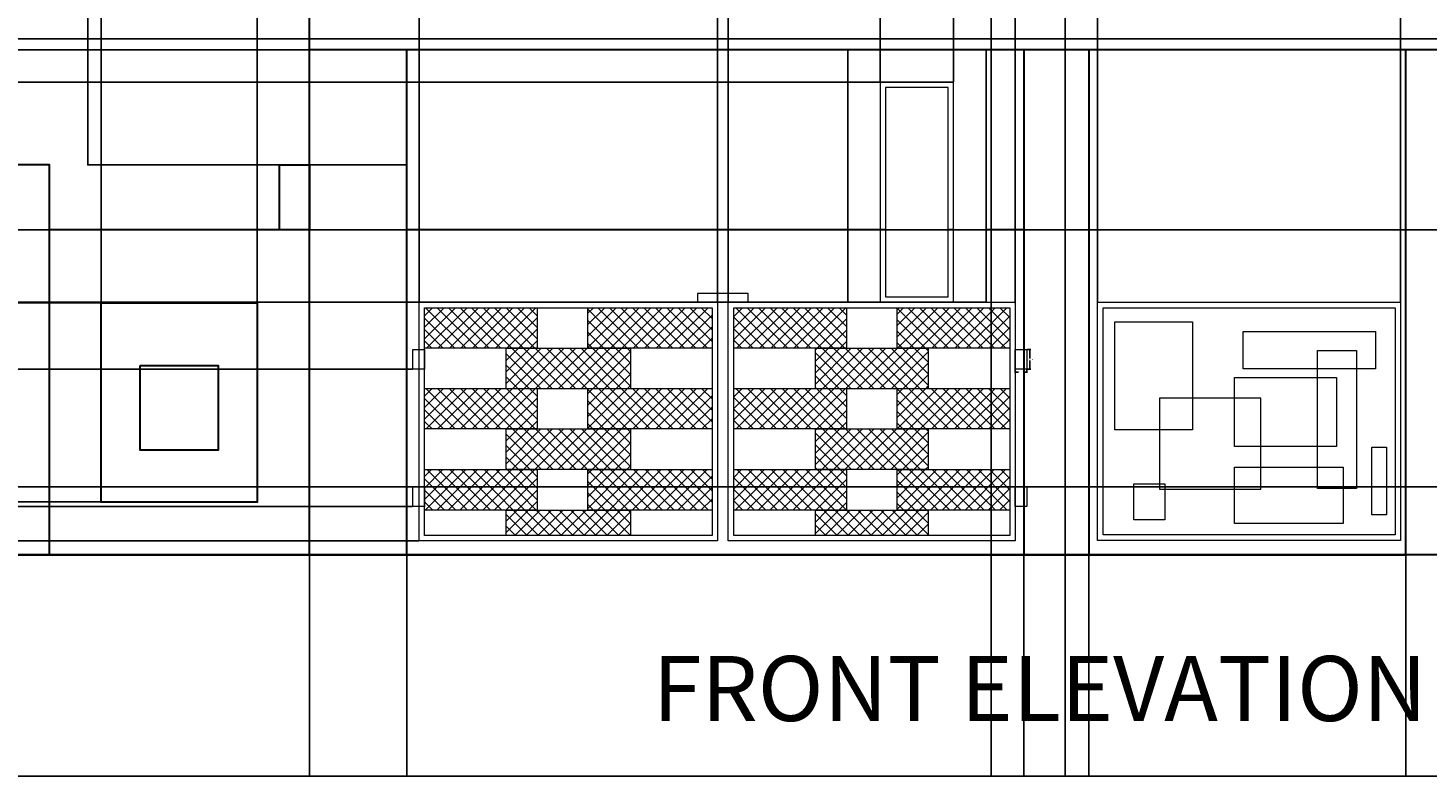
# Model space of a CAD drawing. Units: inches. Extents: x -14 to 886, y 45 to 435.
# Tile 2 of 5: x 125 to 384, y 45 to 184. Entities that reach past the tile are written whole.
import ezdxf

# ---------------------------------------------------------------- set-up
doc = ezdxf.new("R2010")
doc.units = ezdxf.units.IN
doc.header["$MEASUREMENT"] = 0
for name, color, linetype, lineweight in [('A-ANNO-DIMS', 2, 'Continuous', 18), ('A-ANNO-TEXT', 7, 'Continuous', 25), ('A-ELEV-BAND', 7, 'Continuous', 30), ('A-GLAZ', 4, 'Continuous', 18), ('A-WALL', 7, 'Continuous', 25), ('L-GATE', 3, 'Continuous', 18), ('L-GATE-PATT', 252, 'Continuous', 13), ('L-WALL', 7, 'Continuous', 30)]:
    doc.layers.add(name, color=color, linetype=linetype, lineweight=lineweight)
doc.styles.get("Standard").update_dxf_attribs({"font": 'arial.ttf'})
doc.dimstyles.get("Standard").update_dxf_attribs({"dimtxt": 0.18, "dimasz": 0.18, "dimexe": 0.18, "dimexo": 0.0625, "dimgap": 0.09, "dimtad": 0, "dimtih": 1, "dimtoh": 1, "dimdec": 4, "dimzin": 0, "dimdsep": 46, "dimtxsty": 'Standard', "dimcen": 0.09, "dimadec": 0, "dimazin": 0, "dimtfac": 1, "dimtdec": 4, "dimtofl": 0, "dimtmove": 0, "dimatfit": 3, "dimfxl": 1, "dimtolj": 1, "dimtzin": 0, "dimarcsym": 0})
pattern_1 = [(45, (2.113, 0), (-1.06066, 1.06066), []), (135, (2.113, 0), (-1.06066, -1.06066), [])]

# ---------------------------------------------------------------- blocks, each defined once
blk = doc.blocks.new('GATE-HINGE')
blk.add_lwpolyline([(0, 3.59), (2.16, 3.59), (2.16, 0), (0, 0)], close=True)
blk = doc.blocks.new('*D8')
at = {"layer": 'A-ANNO-DIMS', "color": 0, "lineweight": -2, "transparency": 16777216}
for p, q in [((309.89, 124.41), (310.55, 124.41)), ((310.37, 124.23), (310.37, 122.8)), ((310.37, 121), (310.37, 122.43)), ((309.89, 120.82), (310.55, 120.82))]:
    blk.add_line(p, q, dxfattribs=at)
at = {"layer": 'A-ANNO-DIMS', "color": 0, "transparency": 16777216}
for points in [[(310.34, 124.23), (310.4, 124.23), (310.37, 124.41)], [(310.34, 121), (310.4, 121), (310.37, 120.82)]]:
    blk.add_solid(points, dxfattribs=at)
at = {"layer": 'Defpoints', "color": 0, "transparency": 16777216}
for p in [(309.83, 124.41), (310.37, 124.41), (309.83, 120.82)]:
    blk.add_point(p, dxfattribs=at)
at = {"layer": 'A-ANNO-DIMS', "color": 0, "transparency": 16777216, "insert": (310.37, 122.61), "char_height": 0.18, "attachment_point": 5}
blk.add_mtext('\\A1;HINGE 4 TYP.', dxfattribs=at)
blk = doc.blocks.new('*D9')
at = {"layer": 'A-ANNO-DIMS', "color": 0, "lineweight": -2, "transparency": 16777216}
for p, q in [((307.67, 120.75), (307.67, 120.1)), ((307.85, 120.28), (308.29, 120.28)), ((309.65, 120.28), (309.21, 120.28)), ((309.83, 120.75), (309.83, 120.1))]:
    blk.add_line(p, q, dxfattribs=at)
at = {"layer": 'A-ANNO-DIMS', "color": 0, "transparency": 16777216}
for points in [[(307.85, 120.31), (307.85, 120.25), (307.67, 120.28)], [(309.65, 120.31), (309.65, 120.25), (309.83, 120.28)]]:
    blk.add_solid(points, dxfattribs=at)
at = {"layer": 'Defpoints', "color": 0, "transparency": 16777216}
for p in [(307.67, 120.82), (309.83, 120.82), (309.83, 120.28)]:
    blk.add_point(p, dxfattribs=at)
at = {"layer": 'A-ANNO-DIMS', "color": 0, "transparency": 16777216, "insert": (308.75, 120.28), "char_height": 0.18, "attachment_point": 5}
blk.add_mtext('\\A1;2 TYP.', dxfattribs=at)
blk = doc.blocks.new('*D16')
at = {"layer": 'A-ANNO-DIMS', "color": 0, "lineweight": -2, "transparency": 16777216}
for p, q in [((111.3, 86.48), (111.3, 45.47)), ((591.3, 86.48), (591.3, 45.47)), ((111.48, 45.65), (351.01, 45.65)), ((591.12, 45.65), (351.59, 45.65))]:
    blk.add_line(p, q, dxfattribs=at)
at = {"layer": 'A-ANNO-DIMS', "color": 0, "transparency": 16777216}
for points in [[(111.48, 45.68), (111.48, 45.62), (111.3, 45.65)], [(591.12, 45.68), (591.12, 45.62), (591.3, 45.65)]]:
    blk.add_solid(points, dxfattribs=at)
at = {"layer": 'Defpoints', "color": 0, "transparency": 16777216}
for p in [(111.3, 86.54), (591.3, 86.54), (591.3, 45.65)]:
    blk.add_point(p, dxfattribs=at)
at = {"layer": 'A-ANNO-DIMS', "color": 0, "transparency": 16777216, "insert": (351.3, 45.65), "char_height": 0.18, "attachment_point": 5}
blk.add_mtext('\\A1;480', dxfattribs=at)
blk = doc.blocks.new('*D17')
at = {"layer": 'A-ANNO-DIMS', "color": 0, "lineweight": -2, "transparency": 16777216}
for p, q in [((364.17, 393.98), (-13.96, 393.98)), ((-13.78, 393.8), (-13.78, 240.44)), ((-13.78, 86.72), (-13.78, 240.08)), ((111.24, 86.54), (-13.96, 86.54))]:
    blk.add_line(p, q, dxfattribs=at)
at = {"layer": 'A-ANNO-DIMS', "color": 0, "transparency": 16777216}
for points in [[(-13.81, 393.8), (-13.75, 393.8), (-13.78, 393.98)], [(-13.81, 86.72), (-13.75, 86.72), (-13.78, 86.54)]]:
    blk.add_solid(points, dxfattribs=at)
at = {"layer": 'Defpoints', "color": 0, "transparency": 16777216}
for p in [(-13.78, 393.98), (364.23, 393.98), (111.3, 86.54)]:
    blk.add_point(p, dxfattribs=at)
at = {"layer": 'A-ANNO-DIMS', "color": 0, "transparency": 16777216, "insert": (-13.78, 240.26), "char_height": 0.18, "attachment_point": 5}
blk.add_mtext('\\A1;307.44', dxfattribs=at)
blk = doc.blocks.new('*D18')
at = {"layer": 'A-ANNO-DIMS', "color": 0, "lineweight": -2, "transparency": 16777216}
for p, q in [((111.3, 86.48), (111.3, 45.47)), ((177.3, 86.48), (177.3, 45.47)), ((111.48, 45.65), (144.08, 45.65)), ((177.12, 45.65), (144.52, 45.65))]:
    blk.add_line(p, q, dxfattribs=at)
at = {"layer": 'A-ANNO-DIMS', "color": 0, "transparency": 16777216}
for points in [[(111.48, 45.68), (111.48, 45.62), (111.3, 45.65)], [(177.12, 45.68), (177.12, 45.62), (177.3, 45.65)]]:
    blk.add_solid(points, dxfattribs=at)
at = {"layer": 'Defpoints', "color": 0, "transparency": 16777216}
for p in [(111.3, 86.54), (177.3, 86.54), (177.3, 45.65)]:
    blk.add_point(p, dxfattribs=at)
at = {"layer": 'A-ANNO-DIMS', "color": 0, "transparency": 16777216, "insert": (144.3, 45.65), "char_height": 0.18, "attachment_point": 5}
blk.add_mtext('\\A1;66', dxfattribs=at)
blk = doc.blocks.new('*D19')
at = {"layer": 'A-ANNO-DIMS', "color": 0, "lineweight": -2, "transparency": 16777216}
for p, q in [((177.3, 86.48), (177.3, 45.47)), ((195.3, 86.48), (195.3, 45.47)), ((177.48, 45.65), (186.09, 45.65)), ((195.12, 45.65), (186.51, 45.65))]:
    blk.add_line(p, q, dxfattribs=at)
at = {"layer": 'A-ANNO-DIMS', "color": 0, "transparency": 16777216}
for points in [[(177.48, 45.68), (177.48, 45.62), (177.3, 45.65)], [(195.12, 45.68), (195.12, 45.62), (195.3, 45.65)]]:
    blk.add_solid(points, dxfattribs=at)
at = {"layer": 'Defpoints', "color": 0, "transparency": 16777216}
for p in [(177.3, 86.54), (195.3, 86.54), (195.3, 45.65)]:
    blk.add_point(p, dxfattribs=at)
at = {"layer": 'A-ANNO-DIMS', "color": 0, "transparency": 16777216, "insert": (186.3, 45.65), "char_height": 0.18, "attachment_point": 5}
blk.add_mtext('\\A1;18', dxfattribs=at)
blk = doc.blocks.new('*D20')
at = {"layer": 'A-ANNO-DIMS', "color": 0, "lineweight": -2, "transparency": 16777216}
for p, q in [((195.3, 86.48), (195.3, 45.47)), ((309.24, 86.48), (309.24, 45.47)), ((195.48, 45.65), (251.82, 45.65)), ((309.06, 45.65), (252.73, 45.65))]:
    blk.add_line(p, q, dxfattribs=at)
at = {"layer": 'A-ANNO-DIMS', "color": 0, "transparency": 16777216}
for points in [[(195.48, 45.68), (195.48, 45.62), (195.3, 45.65)], [(309.06, 45.68), (309.06, 45.62), (309.24, 45.65)]]:
    blk.add_solid(points, dxfattribs=at)
at = {"layer": 'Defpoints', "color": 0, "transparency": 16777216}
for p in [(195.3, 86.54), (309.24, 86.54), (309.24, 45.65)]:
    blk.add_point(p, dxfattribs=at)
at = {"layer": 'A-ANNO-DIMS', "color": 0, "transparency": 16777216, "insert": (252.27, 45.65), "char_height": 0.18, "attachment_point": 5}
blk.add_mtext('\\A1;113.94', dxfattribs=at)
blk = doc.blocks.new('*D21')
at = {"layer": 'A-ANNO-DIMS', "color": 0, "lineweight": -2, "transparency": 16777216}
for p, q in [((309.24, 86.48), (309.24, 45.47)), ((321.24, 86.48), (321.24, 45.47)), ((309.42, 45.65), (315.03, 45.65)), ((321.06, 45.65), (315.45, 45.65))]:
    blk.add_line(p, q, dxfattribs=at)
at = {"layer": 'A-ANNO-DIMS', "color": 0, "transparency": 16777216}
for points in [[(309.42, 45.68), (309.42, 45.62), (309.24, 45.65)], [(321.06, 45.68), (321.06, 45.62), (321.24, 45.65)]]:
    blk.add_solid(points, dxfattribs=at)
at = {"layer": 'Defpoints', "color": 0, "transparency": 16777216}
for p in [(309.24, 86.54), (321.24, 86.54), (321.24, 45.65)]:
    blk.add_point(p, dxfattribs=at)
at = {"layer": 'A-ANNO-DIMS', "color": 0, "transparency": 16777216, "insert": (315.24, 45.65), "char_height": 0.18, "attachment_point": 5}
blk.add_mtext('\\A1;12', dxfattribs=at)
blk = doc.blocks.new('*D22')
at = {"layer": 'A-ANNO-DIMS', "color": 0, "lineweight": -2, "transparency": 16777216}
for p, q in [((321.24, 86.48), (321.24, 45.47)), ((379.79, 86.48), (379.79, 45.47)), ((321.42, 45.65), (350.12, 45.65)), ((379.61, 45.65), (350.91, 45.65))]:
    blk.add_line(p, q, dxfattribs=at)
at = {"layer": 'A-ANNO-DIMS', "color": 0, "transparency": 16777216}
for points in [[(321.42, 45.68), (321.42, 45.62), (321.24, 45.65)], [(379.61, 45.68), (379.61, 45.62), (379.79, 45.65)]]:
    blk.add_solid(points, dxfattribs=at)
at = {"layer": 'Defpoints', "color": 0, "transparency": 16777216}
for p in [(321.24, 86.54), (379.79, 86.54), (379.79, 45.65)]:
    blk.add_point(p, dxfattribs=at)
at = {"layer": 'A-ANNO-DIMS', "color": 0, "transparency": 16777216, "insert": (350.51, 45.65), "char_height": 0.18, "attachment_point": 5}
blk.add_mtext('\\A1;58.55', dxfattribs=at)
blk = doc.blocks.new('*D23')
at = {"layer": 'A-ANNO-DIMS', "color": 0, "lineweight": -2, "transparency": 16777216}
for p, q in [((379.79, 86.48), (379.79, 45.47)), ((391.79, 86.48), (391.79, 45.47)), ((379.97, 45.65), (385.58, 45.65)), ((391.61, 45.65), (386, 45.65))]:
    blk.add_line(p, q, dxfattribs=at)
at = {"layer": 'A-ANNO-DIMS', "color": 0, "transparency": 16777216}
for points in [[(379.97, 45.68), (379.97, 45.62), (379.79, 45.65)], [(391.61, 45.68), (391.61, 45.62), (391.79, 45.65)]]:
    blk.add_solid(points, dxfattribs=at)
at = {"layer": 'Defpoints', "color": 0, "transparency": 16777216}
for p in [(379.79, 86.54), (391.79, 86.54), (391.79, 45.65)]:
    blk.add_point(p, dxfattribs=at)
at = {"layer": 'A-ANNO-DIMS', "color": 0, "transparency": 16777216, "insert": (385.79, 45.65), "char_height": 0.18, "attachment_point": 5}
blk.add_mtext('\\A1;12', dxfattribs=at)
blk = doc.blocks.new('*D24')
at = {"layer": 'A-ANNO-DIMS', "color": 0, "lineweight": -2, "transparency": 16777216}
for p, q in [((136.31, 311.03), (-13.96, 311.03)), ((-13.78, 310.85), (-13.78, 198.97)), ((-13.78, 86.72), (-13.78, 198.6)), ((195.24, 86.54), (-13.96, 86.54))]:
    blk.add_line(p, q, dxfattribs=at)
at = {"layer": 'A-ANNO-DIMS', "color": 0, "transparency": 16777216}
for points in [[(-13.81, 310.85), (-13.75, 310.85), (-13.78, 311.03)], [(-13.81, 86.72), (-13.75, 86.72), (-13.78, 86.54)]]:
    blk.add_solid(points, dxfattribs=at)
at = {"layer": 'Defpoints', "color": 0, "transparency": 16777216}
for p in [(-13.78, 311.03), (136.37, 311.03), (195.3, 86.54)]:
    blk.add_point(p, dxfattribs=at)
at = {"layer": 'A-ANNO-DIMS', "color": 0, "transparency": 16777216, "insert": (-13.78, 198.79), "char_height": 0.18, "attachment_point": 5}
blk.add_mtext('\\A1;224.5', dxfattribs=at)
blk = doc.blocks.new('*D34')
at = {"layer": 'A-ANNO-DIMS', "color": 0, "lineweight": -2, "transparency": 16777216}
for p, q in [((177.3, 179.88), (177.3, 435.05)), ((177.48, 434.87), (285.86, 434.87)), ((395.16, 434.87), (286.79, 434.87)), ((395.34, 179.88), (395.34, 435.05))]:
    blk.add_line(p, q, dxfattribs=at)
at = {"layer": 'A-ANNO-DIMS', "color": 0, "transparency": 16777216}
for points in [[(177.48, 434.9), (177.48, 434.84), (177.3, 434.87)], [(395.16, 434.9), (395.16, 434.84), (395.34, 434.87)]]:
    blk.add_solid(points, dxfattribs=at)
at = {"layer": 'Defpoints', "color": 0, "transparency": 16777216}
for p in [(395.34, 434.87), (177.3, 179.82), (395.34, 179.82)]:
    blk.add_point(p, dxfattribs=at)
at = {"layer": 'A-ANNO-DIMS', "color": 0, "transparency": 16777216, "insert": (286.32, 434.87), "char_height": 0.18, "attachment_point": 5}
blk.add_mtext('\\A1;218.04', dxfattribs=at)
blk = doc.blocks.new('*D35')
at = {"layer": 'A-ANNO-DIMS', "color": 0, "lineweight": -2, "transparency": 16777216}
for p, q in [((395.28, 217.88), (-13.96, 217.88)), ((-13.78, 217.7), (-13.78, 199.03)), ((-13.78, 180), (-13.78, 198.67)), ((395.28, 179.82), (-13.96, 179.82))]:
    blk.add_line(p, q, dxfattribs=at)
at = {"layer": 'A-ANNO-DIMS', "color": 0, "transparency": 16777216}
for points in [[(-13.81, 217.7), (-13.75, 217.7), (-13.78, 217.88)], [(-13.81, 180), (-13.75, 180), (-13.78, 179.82)]]:
    blk.add_solid(points, dxfattribs=at)
at = {"layer": 'Defpoints', "color": 0, "transparency": 16777216}
for p in [(-13.78, 217.88), (395.34, 217.88), (395.34, 179.82)]:
    blk.add_point(p, dxfattribs=at)
at = {"layer": 'A-ANNO-DIMS', "color": 0, "transparency": 16777216, "insert": (-13.78, 198.85), "char_height": 0.18, "attachment_point": 5}
blk.add_mtext('\\A1;38.06', dxfattribs=at)
blk = doc.blocks.new('*D36')
at = {"layer": 'A-ANNO-DIMS', "color": 0, "lineweight": -2, "transparency": 16777216}
for p, q in [((177.24, 179.82), (-13.96, 179.82)), ((-13.78, 179.64), (-13.78, 133.36)), ((-13.78, 86.72), (-13.78, 133)), ((177.24, 86.54), (-13.96, 86.54))]:
    blk.add_line(p, q, dxfattribs=at)
at = {"layer": 'A-ANNO-DIMS', "color": 0, "transparency": 16777216}
for points in [[(-13.81, 179.64), (-13.75, 179.64), (-13.78, 179.82)], [(-13.81, 86.72), (-13.75, 86.72), (-13.78, 86.54)]]:
    blk.add_solid(points, dxfattribs=at)
at = {"layer": 'Defpoints', "color": 0, "transparency": 16777216}
for p in [(-13.78, 179.82), (177.3, 179.82), (177.3, 86.54)]:
    blk.add_point(p, dxfattribs=at)
at = {"layer": 'A-ANNO-DIMS', "color": 0, "transparency": 16777216, "insert": (-13.78, 133.18), "char_height": 0.18, "attachment_point": 5}
blk.add_mtext('\\A1;93.28', dxfattribs=at)
blk = doc.blocks.new('*D37')
at = {"layer": 'A-ANNO-DIMS', "color": 0, "lineweight": -2, "transparency": 16777216}
for p, q in [((129.24, 146.54), (-13.96, 146.54)), ((-13.78, 146.36), (-13.78, 116.72)), ((-13.78, 86.72), (-13.78, 116.36)), ((129.24, 86.54), (-13.96, 86.54))]:
    blk.add_line(p, q, dxfattribs=at)
at = {"layer": 'A-ANNO-DIMS', "color": 0, "transparency": 16777216}
for points in [[(-13.81, 146.36), (-13.75, 146.36), (-13.78, 146.54)], [(-13.81, 86.72), (-13.75, 86.72), (-13.78, 86.54)]]:
    blk.add_solid(points, dxfattribs=at)
at = {"layer": 'Defpoints', "color": 0, "transparency": 16777216}
for p in [(-13.78, 146.54), (129.3, 146.54), (129.3, 86.54)]:
    blk.add_point(p, dxfattribs=at)
at = {"layer": 'A-ANNO-DIMS', "color": 0, "transparency": 16777216, "insert": (-13.78, 116.54), "char_height": 0.18, "attachment_point": 5}
blk.add_mtext('\\A1;60', dxfattribs=at)
blk = doc.blocks.new('*D41')
at = {"layer": 'A-ANNO-DIMS', "color": 0, "lineweight": -2, "transparency": 16777216}
for p, q in [((591.24, 259.14), (-13.96, 259.14)), ((-13.78, 258.96), (-13.78, 203.02)), ((-13.78, 146.72), (-13.78, 202.66)), ((537.19, 146.54), (-13.96, 146.54))]:
    blk.add_line(p, q, dxfattribs=at)
at = {"layer": 'A-ANNO-DIMS', "color": 0, "transparency": 16777216}
for points in [[(-13.81, 258.96), (-13.75, 258.96), (-13.78, 259.14)], [(-13.81, 146.72), (-13.75, 146.72), (-13.78, 146.54)]]:
    blk.add_solid(points, dxfattribs=at)
at = {"layer": 'Defpoints', "color": 0, "transparency": 16777216}
for p in [(-13.78, 259.14), (591.3, 259.14), (537.25, 146.54)]:
    blk.add_point(p, dxfattribs=at)
at = {"layer": 'A-ANNO-DIMS', "color": 0, "transparency": 16777216, "insert": (-13.78, 202.84), "char_height": 0.18, "attachment_point": 5}
blk.add_mtext('\\A1;112.6', dxfattribs=at)
blk = doc.blocks.new('*D44')
at = {"layer": 'A-ANNO-DIMS', "color": 0, "lineweight": -2, "transparency": 16777216}
for p, q in [((197.49, 133.16), (-13.96, 133.16)), ((-13.78, 132.98), (-13.78, 111.31)), ((-13.78, 89.26), (-13.78, 110.94)), ((197.49, 89.08), (-13.96, 89.08))]:
    blk.add_line(p, q, dxfattribs=at)
at = {"layer": 'A-ANNO-DIMS', "color": 0, "transparency": 16777216}
for points in [[(-13.81, 132.98), (-13.75, 132.98), (-13.78, 133.16)], [(-13.81, 89.26), (-13.75, 89.26), (-13.78, 89.08)]]:
    blk.add_solid(points, dxfattribs=at)
at = {"layer": 'Defpoints', "color": 0, "transparency": 16777216}
for p in [(-13.78, 133.16), (197.55, 133.16), (197.55, 89.08)]:
    blk.add_point(p, dxfattribs=at)
at = {"layer": 'A-ANNO-DIMS', "color": 0, "transparency": 16777216, "insert": (-13.78, 111.12), "char_height": 0.18, "attachment_point": 5}
blk.add_mtext('\\A1;44.08', dxfattribs=at)
blk = doc.blocks.new('*D45')
at = {"layer": 'A-ANNO-DIMS', "color": 0, "lineweight": -2, "transparency": 16777216}
for p, q in [((197.55, 133.22), (197.55, 435.05)), ((197.73, 434.87), (224.73, 434.87)), ((252.49, 434.87), (225.49, 434.87)), ((252.67, 133.22), (252.67, 435.05))]:
    blk.add_line(p, q, dxfattribs=at)
at = {"layer": 'A-ANNO-DIMS', "color": 0, "transparency": 16777216}
for points in [[(197.73, 434.9), (197.73, 434.84), (197.55, 434.87)], [(252.49, 434.9), (252.49, 434.84), (252.67, 434.87)]]:
    blk.add_solid(points, dxfattribs=at)
at = {"layer": 'Defpoints', "color": 0, "transparency": 16777216}
for p in [(252.67, 434.87), (197.55, 133.16), (252.67, 133.16)]:
    blk.add_point(p, dxfattribs=at)
at = {"layer": 'A-ANNO-DIMS', "color": 0, "transparency": 16777216, "insert": (225.11, 434.87), "char_height": 0.18, "attachment_point": 5}
blk.add_mtext('\\A1;55.11', dxfattribs=at)
blk = doc.blocks.new('*D46')
at = {"layer": 'A-ANNO-DIMS', "color": 0, "lineweight": -2, "transparency": 16777216}
for p, q in [((254.67, 133.22), (254.67, 435.05)), ((254.85, 434.87), (280.95, 434.87)), ((307.49, 434.87), (281.39, 434.87)), ((307.67, 133.22), (307.67, 435.05))]:
    blk.add_line(p, q, dxfattribs=at)
at = {"layer": 'A-ANNO-DIMS', "color": 0, "transparency": 16777216}
for points in [[(254.85, 434.9), (254.85, 434.84), (254.67, 434.87)], [(307.49, 434.9), (307.49, 434.84), (307.67, 434.87)]]:
    blk.add_solid(points, dxfattribs=at)
at = {"layer": 'Defpoints', "color": 0, "transparency": 16777216}
for p in [(307.67, 434.87), (254.67, 133.16), (307.67, 133.16)]:
    blk.add_point(p, dxfattribs=at)
at = {"layer": 'A-ANNO-DIMS', "color": 0, "transparency": 16777216, "insert": (281.17, 434.87), "char_height": 0.18, "attachment_point": 5}
blk.add_mtext('\\A1;53', dxfattribs=at)
blk = doc.blocks.new('*D47')
at = {"layer": 'A-ANNO-DIMS', "color": 0, "lineweight": -2, "transparency": 16777216}
for p, q in [((322.89, 133.22), (322.89, 435.05)), ((323.07, 434.87), (350.46, 434.87)), ((378.65, 434.87), (351.25, 434.87)), ((378.83, 133.22), (378.83, 435.05))]:
    blk.add_line(p, q, dxfattribs=at)
at = {"layer": 'A-ANNO-DIMS', "color": 0, "transparency": 16777216}
for points in [[(323.07, 434.9), (323.07, 434.84), (322.89, 434.87)], [(378.65, 434.9), (378.65, 434.84), (378.83, 434.87)]]:
    blk.add_solid(points, dxfattribs=at)
at = {"layer": 'Defpoints', "color": 0, "transparency": 16777216}
for p in [(378.83, 434.87), (322.89, 133.16), (378.83, 133.16)]:
    blk.add_point(p, dxfattribs=at)
at = {"layer": 'A-ANNO-DIMS', "color": 0, "transparency": 16777216, "insert": (350.86, 434.87), "char_height": 0.18, "attachment_point": 5}
blk.add_mtext('\\A1;55.94', dxfattribs=at)
blk = doc.blocks.new('*D54')
at = {"layer": 'A-ANNO-DIMS', "color": 0, "lineweight": -2, "transparency": 16777216}
for p, q in [((444.97, 181.83), (-13.96, 181.83)), ((-13.78, 181.65), (-13.78, 164.37)), ((-13.78, 146.72), (-13.78, 164)), ((444.97, 146.54), (-13.96, 146.54))]:
    blk.add_line(p, q, dxfattribs=at)
at = {"layer": 'A-ANNO-DIMS', "color": 0, "transparency": 16777216}
for points in [[(-13.81, 181.65), (-13.75, 181.65), (-13.78, 181.83)], [(-13.81, 146.72), (-13.75, 146.72), (-13.78, 146.54)]]:
    blk.add_solid(points, dxfattribs=at)
at = {"layer": 'Defpoints', "color": 0, "transparency": 16777216}
for p in [(-13.78, 181.83), (445.04, 181.83), (445.04, 146.54)]:
    blk.add_point(p, dxfattribs=at)
at = {"layer": 'A-ANNO-DIMS', "color": 0, "transparency": 16777216, "insert": (-13.78, 164.19), "char_height": 0.18, "attachment_point": 5}
blk.add_mtext('\\A1;35.29', dxfattribs=at)
blk = doc.blocks.new('*D55')
at = {"layer": 'A-ANNO-DIMS', "color": 0, "lineweight": -2, "transparency": 16777216}
for p, q in [((444.97, 265.67), (-13.96, 265.67)), ((-13.78, 265.49), (-13.78, 223.93)), ((-13.78, 182.01), (-13.78, 223.57)), ((444.97, 181.83), (-13.96, 181.83))]:
    blk.add_line(p, q, dxfattribs=at)
at = {"layer": 'A-ANNO-DIMS', "color": 0, "transparency": 16777216}
for points in [[(-13.81, 265.49), (-13.75, 265.49), (-13.78, 265.67)], [(-13.81, 182.01), (-13.75, 182.01), (-13.78, 181.83)]]:
    blk.add_solid(points, dxfattribs=at)
at = {"layer": 'Defpoints', "color": 0, "transparency": 16777216}
for p in [(-13.78, 265.67), (445.04, 265.67), (445.04, 181.83)]:
    blk.add_point(p, dxfattribs=at)
at = {"layer": 'A-ANNO-DIMS', "color": 0, "transparency": 16777216, "insert": (-13.78, 223.75), "char_height": 0.18, "attachment_point": 5}
blk.add_mtext('\\A1;83.84', dxfattribs=at)
blk = doc.blocks.new('*D57')
at = {"layer": 'A-ANNO-DIMS', "color": 0, "lineweight": -2, "transparency": 16777216}
for p, q in [((404, 99.06), (-13.96, 99.06)), ((-13.78, 98.88), (-13.78, 92.98)), ((-13.78, 86.72), (-13.78, 92.62)), ((391.73, 86.54), (-13.96, 86.54))]:
    blk.add_line(p, q, dxfattribs=at)
at = {"layer": 'A-ANNO-DIMS', "color": 0, "transparency": 16777216}
for points in [[(-13.81, 98.88), (-13.75, 98.88), (-13.78, 99.06)], [(-13.81, 86.72), (-13.75, 86.72), (-13.78, 86.54)]]:
    blk.add_solid(points, dxfattribs=at)
at = {"layer": 'Defpoints', "color": 0, "transparency": 16777216}
for p in [(404.07, 99.06), (-13.78, 86.54), (391.79, 86.54)]:
    blk.add_point(p, dxfattribs=at)
at = {"layer": 'A-ANNO-DIMS', "color": 0, "transparency": 16777216, "insert": (-13.78, 92.8), "char_height": 0.18, "attachment_point": 5}
blk.add_mtext('\\A1;12.52', dxfattribs=at)
blk = doc.blocks.new('*D61')
at = {"layer": 'A-ANNO-DIMS', "color": 0, "lineweight": -2, "transparency": 16777216}
for p, q in [((282.73, 173.88), (282.73, 435.05)), ((282.91, 434.87), (289.04, 434.87)), ((296.09, 434.87), (289.96, 434.87)), ((296.27, 173.88), (296.27, 435.05))]:
    blk.add_line(p, q, dxfattribs=at)
at = {"layer": 'A-ANNO-DIMS', "color": 0, "transparency": 16777216}
for points in [[(282.91, 434.9), (282.91, 434.84), (282.73, 434.87)], [(296.09, 434.9), (296.09, 434.84), (296.27, 434.87)]]:
    blk.add_solid(points, dxfattribs=at)
at = {"layer": 'Defpoints', "color": 0, "transparency": 16777216}
for p in [(296.27, 434.87), (282.73, 173.82), (296.27, 173.82)]:
    blk.add_point(p, dxfattribs=at)
at = {"layer": 'A-ANNO-DIMS', "color": 0, "transparency": 16777216, "insert": (289.5, 434.87), "char_height": 0.18, "attachment_point": 5}
blk.add_mtext('\\A1;13.538', dxfattribs=at)
blk = doc.blocks.new('*D62')
at = {"layer": 'A-ANNO-DIMS', "color": 0, "lineweight": -2, "transparency": 16777216}
for p, q in [((296.21, 173.82), (-13.96, 173.82)), ((-13.78, 173.64), (-13.78, 153.67)), ((-13.78, 133.34), (-13.78, 153.31)), ((296.21, 133.16), (-13.96, 133.16))]:
    blk.add_line(p, q, dxfattribs=at)
at = {"layer": 'A-ANNO-DIMS', "color": 0, "transparency": 16777216}
for points in [[(-13.81, 173.64), (-13.75, 173.64), (-13.78, 173.82)], [(-13.81, 133.34), (-13.75, 133.34), (-13.78, 133.16)]]:
    blk.add_solid(points, dxfattribs=at)
at = {"layer": 'Defpoints', "color": 0, "transparency": 16777216}
for p in [(-13.78, 173.82), (296.27, 173.82), (296.27, 133.16)]:
    blk.add_point(p, dxfattribs=at)
at = {"layer": 'A-ANNO-DIMS', "color": 0, "transparency": 16777216, "insert": (-13.78, 153.49), "char_height": 0.18, "attachment_point": 5}
blk.add_mtext('\\A1;40.66', dxfattribs=at)
blk = doc.blocks.new('*D63')
at = {"layer": 'A-ANNO-DIMS', "color": 0, "lineweight": -2, "transparency": 16777216}
for p, q in [((138.83, 133.13), (138.83, 435.05)), ((139.01, 434.87), (152.85, 434.87)), ((167.48, 434.87), (153.64, 434.87)), ((167.66, 133.13), (167.66, 435.05))]:
    blk.add_line(p, q, dxfattribs=at)
at = {"layer": 'A-ANNO-DIMS', "color": 0, "transparency": 16777216}
for points in [[(139.01, 434.9), (139.01, 434.84), (138.83, 434.87)], [(167.48, 434.9), (167.48, 434.84), (167.66, 434.87)]]:
    blk.add_solid(points, dxfattribs=at)
at = {"layer": 'Defpoints', "color": 0, "transparency": 16777216}
for p in [(167.66, 434.87), (138.83, 133.07), (167.66, 133.07)]:
    blk.add_point(p, dxfattribs=at)
at = {"layer": 'A-ANNO-DIMS', "color": 0, "transparency": 16777216, "insert": (153.25, 434.87), "char_height": 0.18, "attachment_point": 5}
blk.add_mtext('\\A1;28.83', dxfattribs=at)
blk = doc.blocks.new('*D64')
at = {"layer": 'A-ANNO-DIMS', "color": 0, "lineweight": -2, "transparency": 16777216}
for p, q in [((138.77, 133.07), (-13.96, 133.07)), ((-13.78, 132.89), (-13.78, 114.85)), ((-13.78, 96.45), (-13.78, 114.49)), ((138.77, 96.27), (-13.96, 96.27))]:
    blk.add_line(p, q, dxfattribs=at)
at = {"layer": 'A-ANNO-DIMS', "color": 0, "transparency": 16777216}
for points in [[(-13.81, 132.89), (-13.75, 132.89), (-13.78, 133.07)], [(-13.81, 96.45), (-13.75, 96.45), (-13.78, 96.27)]]:
    blk.add_solid(points, dxfattribs=at)
at = {"layer": 'Defpoints', "color": 0, "transparency": 16777216}
for p in [(-13.78, 133.07), (138.83, 133.07), (138.83, 96.27)]:
    blk.add_point(p, dxfattribs=at)
at = {"layer": 'A-ANNO-DIMS', "color": 0, "transparency": 16777216, "insert": (-13.78, 114.67), "char_height": 0.18, "attachment_point": 5}
blk.add_mtext('\\A1;36.8', dxfattribs=at)
blk = doc.blocks.new('*D65')
at = {"layer": 'A-ANNO-DIMS', "color": 0, "lineweight": -2, "transparency": 16777216}
for p, q in [((111.3, 158.6), (111.3, 435.05)), ((111.48, 434.87), (123.44, 434.87)), ((136.19, 434.87), (124.23, 434.87)), ((136.37, 158.6), (136.37, 435.05))]:
    blk.add_line(p, q, dxfattribs=at)
at = {"layer": 'A-ANNO-DIMS', "color": 0, "transparency": 16777216}
for points in [[(111.48, 434.9), (111.48, 434.84), (111.3, 434.87)], [(136.19, 434.9), (136.19, 434.84), (136.37, 434.87)]]:
    blk.add_solid(points, dxfattribs=at)
at = {"layer": 'Defpoints', "color": 0, "transparency": 16777216}
for p in [(136.37, 434.87), (111.3, 158.54), (136.37, 158.54)]:
    blk.add_point(p, dxfattribs=at)
at = {"layer": 'A-ANNO-DIMS', "color": 0, "transparency": 16777216, "insert": (123.84, 434.87), "char_height": 0.18, "attachment_point": 5}
blk.add_mtext('\\A1;25.07', dxfattribs=at)
blk = doc.blocks.new('*D66')
at = {"layer": 'A-ANNO-DIMS', "color": 0, "lineweight": -2, "transparency": 16777216}
for p, q in [((303.24, 217.82), (303.24, 45.47)), ((316.91, 217.82), (316.91, 45.47)), ((303.42, 45.65), (309.69, 45.65)), ((316.73, 45.65), (310.46, 45.65))]:
    blk.add_line(p, q, dxfattribs=at)
at = {"layer": 'A-ANNO-DIMS', "color": 0, "transparency": 16777216}
for points in [[(303.42, 45.68), (303.42, 45.62), (303.24, 45.65)], [(316.73, 45.68), (316.73, 45.62), (316.91, 45.65)]]:
    blk.add_solid(points, dxfattribs=at)
at = {"layer": 'Defpoints', "color": 0, "transparency": 16777216}
for p in [(303.24, 217.88), (316.91, 217.88), (316.91, 45.65)]:
    blk.add_point(p, dxfattribs=at)
at = {"layer": 'A-ANNO-DIMS', "color": 0, "transparency": 16777216, "insert": (310.07, 45.65), "char_height": 0.18, "attachment_point": 5}
blk.add_mtext('\\A1;13.67', dxfattribs=at)
blk = doc.blocks.new('*D68')
at = {"layer": 'A-ANNO-DIMS', "color": 0, "lineweight": -2, "transparency": 16777216}
for p, q in [((196.33, 120.82), (-13.96, 120.82)), ((-13.78, 120.64), (-13.78, 108.32)), ((-13.78, 95.64), (-13.78, 107.96)), ((196.33, 95.46), (-13.96, 95.46))]:
    blk.add_line(p, q, dxfattribs=at)
at = {"layer": 'A-ANNO-DIMS', "color": 0, "transparency": 16777216}
for points in [[(-13.81, 120.64), (-13.75, 120.64), (-13.78, 120.82)], [(-13.81, 95.64), (-13.75, 95.64), (-13.78, 95.46)]]:
    blk.add_solid(points, dxfattribs=at)
at = {"layer": 'Defpoints', "color": 0, "transparency": 16777216}
for p in [(-13.78, 120.82), (196.39, 120.82), (196.39, 95.46)]:
    blk.add_point(p, dxfattribs=at)
at = {"layer": 'A-ANNO-DIMS', "color": 0, "transparency": 16777216, "insert": (-13.78, 108.14), "char_height": 0.18, "attachment_point": 5}
blk.add_mtext('\\A1;25.356', dxfattribs=at)

msp = doc.modelspace()

# ---------------------------------------------------------------- hatches: boundary and pattern name
at = {"layer": 'L-GATE-PATT'}
h = msp.add_hatch(dxfattribs=at)
h.set_pattern_fill('ANSI37', color=256, scale=12)
h.paths.add_polyline_path([(198.5542, 132.1624), (198.5542, 124.6655), (219.3809, 124.6655), (219.3809, 132.1624)])
h.paths.add_polyline_path([(228.7275, 132.1624), (228.7275, 124.6655), (251.6671, 124.6655), (251.6671, 132.1624)])
h.paths.add_polyline_path([(228.7275, 117.2617), (236.5805, 117.2617), (236.5805, 124.6655), (213.6409, 124.6655), (213.6409, 117.2617), (219.3809, 117.2617), (228.7275, 117.2111)])
h.paths.add_polyline_path([(219.3809, 109.7648), (219.3809, 117.1686), (213.6409, 117.1686), (198.5542, 117.2617), (198.5542, 109.7648)])
h.paths.add_polyline_path([(236.5805, 117.2617), (236.5805, 117.1686), (228.7275, 117.1686), (228.7275, 109.7648), (251.6671, 109.7648), (251.6671, 117.2617)])
h.paths.add_polyline_path([(213.6409, 109.7648), (213.6409, 102.2678), (236.5805, 102.2678), (236.5805, 109.7648)])
h.paths.add_polyline_path([(198.5542, 102.2513), (198.5542, 94.7543), (219.3809, 94.7543), (219.3809, 102.2513)])
h.paths.add_polyline_path([(228.7275, 102.2513), (228.7275, 94.7543), (251.6671, 94.7543), (251.6671, 102.2513)])
h.paths.add_polyline_path([(213.6409, 94.7543), (213.6409, 90.0847), (236.5805, 90.0847), (236.5805, 94.7543)])
h = msp.add_hatch(dxfattribs=at)
h.set_pattern_fill('ANSI37', color=256, scale=12)
h.set_pattern_definition(pattern_1)
h.paths.add_polyline_path([(255.6671, 132.1624), (255.6671, 124.6655), (276.4938, 124.6655), (276.4938, 132.1624)])
h.paths.add_polyline_path([(306.6671, 124.6655), (306.6671, 132.1624), (285.8405, 132.1624), (285.8405, 124.6655)])
h.paths.add_polyline_path([(270.7538, 124.6655), (270.7538, 117.2617), (276.4938, 117.2617), (285.8405, 117.204), (285.8405, 117.2617), (291.5805, 117.2617), (291.5805, 124.6655)])
h.paths.add_polyline_path([(255.6671, 117.2617), (255.6671, 109.7648), (276.4938, 109.7648), (276.4938, 117.1686), (270.7538, 117.1686)])
h.paths.add_polyline_path([(291.5805, 117.2617), (291.5805, 117.1686), (285.8405, 117.1686), (285.8405, 109.7648), (306.6671, 109.7648), (306.6671, 117.2617)])
h.paths.add_polyline_path([(270.7538, 109.7648), (270.7538, 102.2678), (291.5805, 102.2678), (291.5805, 109.7648)])
h.paths.add_polyline_path([(255.6671, 102.2513), (255.6671, 94.7543), (276.4938, 94.7543), (276.4938, 102.2513)])
h.paths.add_polyline_path([(306.6671, 94.7543), (306.6671, 102.2513), (285.8405, 102.2513), (285.8405, 94.7543)])
h = msp.add_hatch(dxfattribs=at)
h.set_pattern_fill('ANSI37', color=256, scale=12)
h.set_pattern_definition(pattern_1)
h.paths.add_polyline_path([(270.7538, 94.7543), (270.7538, 90.0847), (291.5805, 90.0847), (291.5805, 94.7543)])

# ---------------------------------------------------------------- linework, layer by layer
at = {"layer": 'A-ELEV-BAND'}
msp.add_lwpolyline([(379.7908, 217.8839), (379.7908, 319.7815), (309.2386, 319.7815), (309.2386, 217.8839), (395.3394, 217.8839), (395.3394, 179.8201), (177.3024, 179.8201)], dxfattribs=at)
at = {"layer": 'A-GLAZ'}
for points in [[(282.7312, 133.1624), (296.2693, 133.1624), (296.2693, 173.8201), (282.7312, 173.8201)], [(283.7312, 134.1624), (295.2693, 134.1624), (295.2693, 172.8201), (283.7312, 172.8201)]]:
    msp.add_lwpolyline(points, close=True, dxfattribs=at)
at = {"layer": 'A-WALL'}
msp.add_lwpolyline([(136.3714, 194.5389), (136.3714, 158.5389), (195.3024, 158.5389)], dxfattribs=at)
msp.add_lwpolyline([(276.7312, 133.1624), (302.2693, 133.1624), (302.2693, 179.8201), (276.7312, 179.8201)], close=True, dxfattribs=at)
at = {"layer": 'L-GATE'}
for points in [[(249.0045, 133.1624), (258.3557, 133.1624), (258.3557, 134.7893), (249.0045, 134.7893)], [(252.6671, 89.0847), (197.5542, 89.0847), (197.5542, 133.1624), (252.6671, 133.1624)], [(251.6671, 90.0847), (198.5542, 90.0847), (198.5542, 132.1624), (251.6671, 132.1624)], [(198.5542, 132.1624), (219.3809, 132.1624), (219.3809, 124.6655), (198.5542, 124.6655)], [(228.7275, 132.1624), (251.6671, 132.1624), (251.6671, 124.6655), (228.7275, 124.6655)], [(254.6671, 133.1624), (307.6671, 133.1624), (307.6671, 89.0847), (254.6671, 89.0847)], [(255.6671, 132.1624), (306.6671, 132.1624), (306.6671, 90.0847), (255.6671, 90.0847)], [(255.6671, 132.1624), (276.4938, 132.1624), (276.4938, 124.6655), (255.6671, 124.6655)], [(285.8405, 132.1624), (306.6671, 132.1624), (306.6671, 124.6655), (285.8405, 124.6655)], [(322.8853, 133.1624), (378.8292, 133.1624), (378.8292, 89.1769), (322.8853, 89.1769)], [(323.8853, 132.1624), (377.8292, 132.1624), (377.8292, 90.1769), (323.8853, 90.1769)], [(326.0546, 129.5489), (340.4332, 129.5489), (340.4332, 109.6273), (326.0546, 109.6273)], [(349.7928, 127.7871), (374.2092, 127.7871), (374.2092, 120.8755), (349.7928, 120.8755)], [(213.6409, 124.6655), (236.5805, 124.6655), (236.5805, 117.1686), (213.6409, 117.1686)], [(270.7538, 124.6655), (291.5805, 124.6655), (291.5805, 117.1686), (270.7538, 117.1686)], [(363.4931, 124.2636), (370.6824, 124.2636), (370.6824, 98.7856), (363.4931, 98.7856)], [(348.165, 119.2493), (367.02, 119.2493), (367.02, 106.5103), (348.165, 106.5103)], [(198.5542, 117.2617), (219.3809, 117.2617), (219.3809, 109.7648), (198.5542, 109.7648)], [(228.7275, 117.2617), (251.6671, 117.2617), (251.6671, 109.7648), (228.7275, 109.7648)], [(255.6671, 117.2617), (276.4938, 117.2617), (276.4938, 109.7648), (255.6671, 109.7648)], [(285.8405, 117.2617), (306.6671, 117.2617), (306.6671, 109.7648), (285.8405, 109.7648)], [(334.329, 98.65), (353.0483, 98.65), (353.0483, 115.4547), (334.329, 115.4547)], [(213.6409, 109.7648), (236.5805, 109.7648), (236.5805, 102.2678), (213.6409, 102.2678)], [(270.7538, 109.7648), (291.5805, 109.7648), (291.5805, 102.2678), (270.7538, 102.2678)], [(373.531, 106.3748), (376.2439, 106.3748), (376.2439, 93.9068), (373.531, 93.9068)], [(198.5542, 102.2513), (219.3809, 102.2513), (219.3809, 94.7543), (198.5542, 94.7543)], [(228.7275, 102.2513), (251.6671, 102.2513), (251.6671, 94.7543), (228.7275, 94.7543)], [(255.6671, 102.2513), (276.4938, 102.2513), (276.4938, 94.7543), (255.6671, 94.7543)], [(285.8405, 102.2513), (306.6671, 102.2513), (306.6671, 94.7543), (285.8405, 94.7543)], [(348.165, 102.7157), (368.2408, 102.7157), (368.2408, 92.2805), (348.165, 92.2805)], [(329.5814, 99.5987), (335.2786, 99.5987), (335.2786, 92.9581), (329.5814, 92.9581)]]:
    msp.add_lwpolyline(points, close=True, dxfattribs=at)
for points in [[(213.6409, 90.0847), (213.6409, 94.7543), (236.5805, 94.7543), (236.5805, 90.0847)], [(270.7538, 90.0847), (270.7538, 94.7543), (291.5805, 94.7543), (291.5805, 90.0847)]]:
    msp.add_lwpolyline(points, dxfattribs=at)
at = {"layer": 'L-WALL'}
for p, q in [((177.3024, 86.5389), (177.3024, 194.5389)), ((195.3024, 86.5389), (195.3024, 179.8201)), ((309.2386, 179.8201), (309.2386, 86.5389)), ((321.2386, 179.8201), (321.2386, 86.5389)), ((177.3024, 146.5389), (129.3024, 146.5389)), ((283.7312, 146.5389), (195.3024, 146.5389)), ((296.2693, 146.5389), (295.2693, 146.5389)), ((309.2386, 146.5389), (302.2693, 146.5389)), ((591.3024, 86.5389), (379.7908, 86.5389))]:
    msp.add_line(p, q, dxfattribs=at)
msp.add_lwpolyline([(129.3024, 86.5389), (129.3024, 158.5389), (111.3024, 158.5389), (111.3024, 86.5389), (379.7908, 86.5389), (379.7908, 179.8201)], dxfattribs=at)
for points in [[(177.3024, 146.5389), (171.7994, 146.5389), (171.7994, 158.5389), (177.3024, 158.5389)], [(138.8348, 133.0686), (167.6621, 133.0686), (167.6621, 96.2677), (138.8348, 96.2677)], [(146.0416, 121.4683), (160.4553, 121.4683), (160.4553, 105.868), (146.0416, 105.868)]]:
    msp.add_lwpolyline(points, close=True, dxfattribs=at)

# ---------------------------------------------------------------- block references
at = {"layer": 'L-GATE'}
for p in [(196.3935, 120.8171), (307.6671, 120.8171), (196.3935, 95.4612), (307.6671, 95.4612)]:
    msp.add_blockref('GATE-HINGE', p, dxfattribs=at)

# ---------------------------------------------------------------- texts
at = {"layer": 'A-ANNO-TEXT'}
msp.add_text('FRONT ELEVATION', height=12, dxfattribs=at).set_placement((240.686, 55.8141))

# ---------------------------------------------------------------- dimensions: what is measured, and where the dimension line sits
at = {"layer": 'A-ANNO-DIMS'}
for base, p1, p2, override, picture, middle in [((136.3714, 434.8697), (111.3024, 158.5389), (136.3714, 158.5389), {"dimdec": 2, "dimlfac": 1, "dimrnd": 0, "dimzin": 0, "dimdsep": 46, "dimlunit": 2}, '*D65', (123.8369, 434.8697)), ((167.6621, 434.8697), (138.8348, 133.0686), (167.6621, 133.0686), {"dimdec": 2, "dimlfac": 1, "dimrnd": 0, "dimzin": 0, "dimdsep": 46, "dimlunit": 2}, '*D63', (153.2485, 434.8697)), ((395.3394, 434.8697), (177.3024, 179.8201), (395.3394, 179.8201), {"dimdec": 2, "dimlfac": 1, "dimrnd": 0, "dimzin": 0, "dimdsep": 46, "dimlunit": 2}, '*D34', (286.3209, 434.8697)), ((252.6671, 434.8697), (197.5542, 133.1624), (252.6671, 133.1624), {"dimdec": 2, "dimlfac": 1, "dimrnd": 0, "dimzin": 0, "dimdsep": 46, "dimlunit": 2}, '*D45', (225.1107, 434.8697)), ((307.6671, 434.8697), (254.6671, 133.1624), (307.6671, 133.1624), {"dimdec": 0, "dimlfac": 1, "dimrnd": 0, "dimzin": 0, "dimdsep": 46, "dimlunit": 2}, '*D46', (281.1671, 434.8697)), ((296.2693, 434.8697), (282.7312, 173.8201), (296.2693, 173.8201), {"dimdec": 3, "dimlfac": 1, "dimrnd": 0, "dimzin": 0, "dimdsep": 46, "dimlunit": 2}, '*D61', (289.5003, 434.8697)), ((378.8292, 434.8697), (322.8853, 133.1624), (378.8292, 133.1624), {"dimdec": 2, "dimlfac": 1, "dimrnd": 0, "dimzin": 0, "dimdsep": 46, "dimlunit": 2}, '*D47', (350.8573, 434.8697)), ((316.9091, 45.6489), (303.2386, 217.8839), (316.9091, 217.8839), {"dimdec": 2, "dimlfac": 1, "dimrnd": 0, "dimzin": 0, "dimdsep": 46, "dimlunit": 2}, '*D66', (310.0739, 45.6489)), ((591.3024, 45.6489), (111.3024, 86.5389), (591.3024, 86.5389), {"dimdec": 0, "dimlfac": 1, "dimrnd": 0, "dimzin": 0, "dimdsep": 46, "dimlunit": 2}, '*D16', (351.3024, 45.6489)), ((177.3024, 45.6489), (111.3024, 86.5389), (177.3024, 86.5389), {"dimdec": 0, "dimlfac": 1, "dimrnd": 0, "dimzin": 0, "dimdsep": 46, "dimlunit": 2}, '*D18', (144.3024, 45.6489)), ((195.3024, 45.6489), (177.3024, 86.5389), (195.3024, 86.5389), {"dimdec": 0, "dimlfac": 1, "dimrnd": 0, "dimzin": 0, "dimdsep": 46, "dimlunit": 2}, '*D19', (186.3024, 45.6489)), ((309.2386, 45.6489), (195.3024, 86.5389), (309.2386, 86.5389), {"dimdec": 2, "dimlfac": 1, "dimrnd": 0, "dimzin": 0, "dimdsep": 46, "dimlunit": 2}, '*D20', (252.2705, 45.6489)), ((321.2386, 45.6489), (309.2386, 86.5389), (321.2386, 86.5389), {"dimdec": 0, "dimlfac": 1, "dimrnd": 0, "dimzin": 0, "dimdsep": 46, "dimlunit": 2}, '*D21', (315.2386, 45.6489)), ((379.7908, 45.6489), (321.2386, 86.5389), (379.7908, 86.5389), {"dimdec": 2, "dimlfac": 1, "dimrnd": 0, "dimzin": 0, "dimdsep": 46, "dimlunit": 2}, '*D22', (350.5147, 45.6489)), ((391.7908, 45.6489), (379.7908, 86.5389), (391.7908, 86.5389), {"dimdec": 0, "dimlfac": 1, "dimrnd": 0, "dimzin": 0, "dimdsep": 46, "dimlunit": 2}, '*D23', (385.7908, 45.6489))]:
    dim = msp.add_linear_dim(base=base, p1=p1, p2=p2, dimstyle='Standard', override=override, dxfattribs=at)
    dim.commit()
    dim.dimension.update_dxf_attribs({"geometry": picture, "text_midpoint": middle})
for base, p1, p2, override, picture, middle in [((-13.7769, 393.9797), (111.3024, 86.5389), (364.2304, 393.9797), {"dimdec": 2, "dimlfac": 1, "dimrnd": 0, "dimzin": 0, "dimdsep": 46, "dimlunit": 2}, '*D17', (-13.7769, 240.2593)), ((-13.7769, 311.0336), (195.3024, 86.5389), (136.3714, 311.0336), {"dimdec": 1, "dimlfac": 1, "dimrnd": 0, "dimzin": 0, "dimdsep": 46, "dimlunit": 2}, '*D24', (-13.7769, 198.7862)), ((-13.7769, 265.6686), (445.0372, 181.8319), (445.0372, 265.6686), {"dimdec": 2, "dimlfac": 1, "dimrnd": 0, "dimzin": 0, "dimdsep": 46, "dimlunit": 2}, '*D55', (-13.7769, 223.7503)), ((-13.7769, 259.1435), (537.2506, 146.5389), (591.3024, 259.1435), {"dimdec": 1, "dimlfac": 1, "dimrnd": 0, "dimzin": 0, "dimdsep": 46, "dimlunit": 2}, '*D41', (-13.7769, 202.8412)), ((-13.7769, 217.8839), (395.3394, 179.8201), (395.3394, 217.8839), {"dimdec": 2, "dimlfac": 1, "dimrnd": 0, "dimzin": 0, "dimdsep": 46, "dimlunit": 2}, '*D35', (-13.7769, 198.852)), ((-13.7769, 181.8319), (445.0372, 146.5389), (445.0372, 181.8319), {"dimdec": 2, "dimlfac": 1, "dimrnd": 0, "dimzin": 0, "dimdsep": 46, "dimlunit": 2}, '*D54', (-13.7769, 164.1854)), ((-13.7769, 179.8201), (177.3024, 86.5389), (177.3024, 179.8201), {"dimdec": 2, "dimlfac": 1, "dimrnd": 0, "dimzin": 0, "dimdsep": 46, "dimlunit": 2}, '*D36', (-13.7769, 133.1795)), ((-13.7769, 173.8201), (296.2693, 133.1624), (296.2693, 173.8201), {"dimdec": 2, "dimlfac": 1, "dimrnd": 0, "dimzin": 0, "dimdsep": 46, "dimlunit": 2}, '*D62', (-13.7769, 153.4913)), ((-13.7769, 146.5389), (129.3024, 86.5389), (129.3024, 146.5389), {"dimdec": 0, "dimlfac": 1, "dimrnd": 0, "dimzin": 0, "dimdsep": 46, "dimlunit": 2}, '*D37', (-13.7769, 116.5389)), ((-13.7769, 133.1624), (197.5542, 89.0847), (197.5542, 133.1624), {"dimdec": 2, "dimlfac": 1, "dimrnd": 0, "dimzin": 0, "dimdsep": 46, "dimlunit": 2}, '*D44', (-13.7769, 111.1236)), ((-13.7769, 133.0686), (138.8348, 96.2677), (138.8348, 133.0686), {"dimdec": 1, "dimlfac": 1, "dimrnd": 0, "dimzin": 0, "dimdsep": 46, "dimlunit": 2}, '*D64', (-13.7769, 114.6682)), ((-13.7769, 120.8171), (196.3935, 95.4612), (196.3935, 120.8171), {"dimdec": 3, "dimlfac": 1, "dimrnd": 0, "dimzin": 0, "dimdsep": 46, "dimlunit": 2}, '*D68', (-13.7769, 108.1391)), ((-13.7769, 86.5389), (404.0655, 99.0583), (391.7908, 86.5389), {"dimdec": 2, "dimlfac": 1, "dimrnd": 0, "dimzin": 0, "dimdsep": 46, "dimlunit": 2}, '*D57', (-13.7769, 92.7986))]:
    dim = msp.add_linear_dim(base=base, p1=p1, p2=p2, angle=90, dimstyle='Standard', override=override, dxfattribs=at)
    dim.commit()
    dim.dimension.update_dxf_attribs({"geometry": picture, "text_midpoint": middle})
dim = msp.add_linear_dim(base=(310.3669, 124.4111), p1=(309.8278, 120.8171), p2=(309.8278, 124.4111), angle=90, text='HINGE <> TYP.', dimstyle='Standard', override={"dimdec": 0, "dimlfac": 1, "dimrnd": 0, "dimzin": 0, "dimdsep": 46, "dimlunit": 2}, dxfattribs=at)
dim.commit()
dim.dimension.update_dxf_attribs({"geometry": '*D8', "text_midpoint": (310.3669, 122.6141)})
dim = msp.add_linear_dim(base=(309.8278, 120.2779), p1=(307.6671, 120.8171), p2=(309.8278, 120.8171), text='<> TYP.', dimstyle='Standard', override={"dimdec": 0, "dimlfac": 1, "dimrnd": 0, "dimzin": 0, "dimdsep": 46, "dimlunit": 2}, dxfattribs=at)
dim.commit()
dim.dimension.update_dxf_attribs({"geometry": '*D9', "text_midpoint": (308.7475, 120.2779)})

doc.saveas('drawing.dxf')
